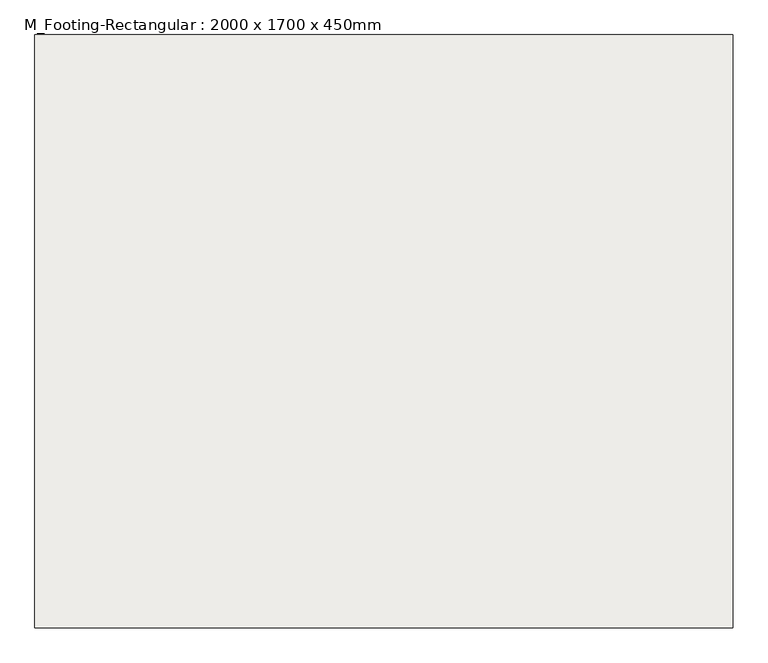
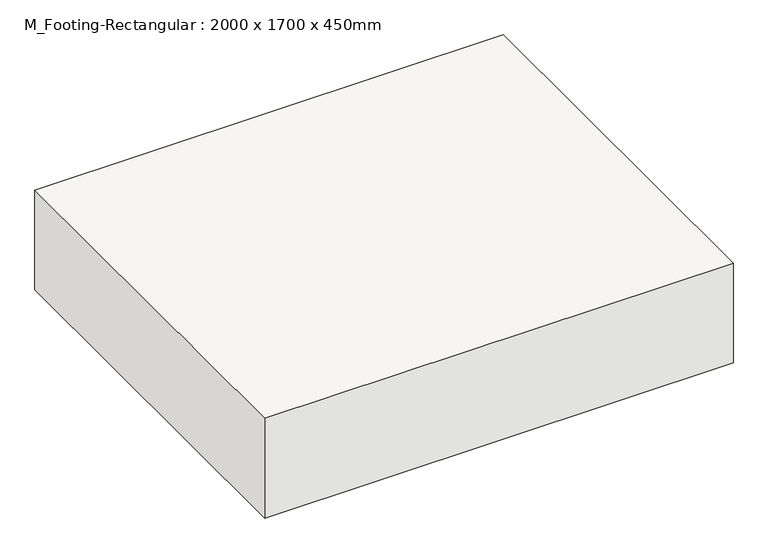
"""IFC4 building model written with IfcOpenShell, lengths in millimetres: slab geometry, M_Footing-Rectangular : 2000 x 1700 x 450mm."""

from ifc_helpers import new_model, si_unit, frame, origin, place, context, project, spatial, polyline, outline, extrude, source, transform, mapped, element, save


def m_footing_rectangular_2000_x_1700_x_450mm_1621679d(model_context):
    return source(origin(), model_context, "Body", "SweptSolid", [
        extrude(outline(polyline([(1000.0, 850.0), (1000.0, -850.0), (-1000.0, -850.0), (-1000.0, 850.0), (1000.0, 850.0)])), frame((0.0, 0.0, -450.0), z_axis=(0.0, 0.0, 1.0), x_axis=(1.0, 0.0, 0.0)), (0.0, 0.0, 1.0), 450.0),
    ])


if __name__ == "__main__":
    model = new_model("IFC4")
    model_context = context("Model", 3, world=origin())
    ifc_project = project(units=[si_unit("LENGTHUNIT", "METRE", prefix="MILLI")], contexts=[model_context])
    site = spatial("IfcSite", under=ifc_project)
    building = spatial("IfcBuilding", under=site)
    placement = place(None, origin())
    m_footing_rectangular_2000_x_1700_x_450mm_shape = m_footing_rectangular_2000_x_1700_x_450mm_1621679d(model_context)
    element("IfcSlab", 1, ObjectType="M_Footing-Rectangular : 2000 x 1700 x 450mm", at=placement, inside=building, context=model_context, shape_type="MappedRepresentation", body=[
        mapped(m_footing_rectangular_2000_x_1700_x_450mm_shape, transform((0.0, 0.0, 0.0), x_axis=(1.0, 0.0, 0.0), y_axis=(0.0, 1.0, 0.0), z_axis=(0.0, 0.0, 1.0))),
    ])
    save(model, "model.ifc")

# Revit data of these elements
# Type "M_Footing-Rectangular : 2000 x 1700 x 450mm"
#   Width = 6' - 6.74016"
#   Length = 5' - 6.92913"
#   Foundation Thickness = 1' - 5.71654"
#   Structural Material [instance default] = Concrete, Cast-in-Place gray
#   Assembly Code = ""
# Element 1 (IfcSlab, "M_Footing-Rectangular : 2000 x 1700 x 450mm")
#   Materials on its faces: "Concrete, Cast-in-Place gray"
# Materials
#   "Concrete, Cast-in-Place gray": class "Concrete", colour RGB 192 192 192, transparency 0, Description = "Cast-in-place concrete", Cost = 0
